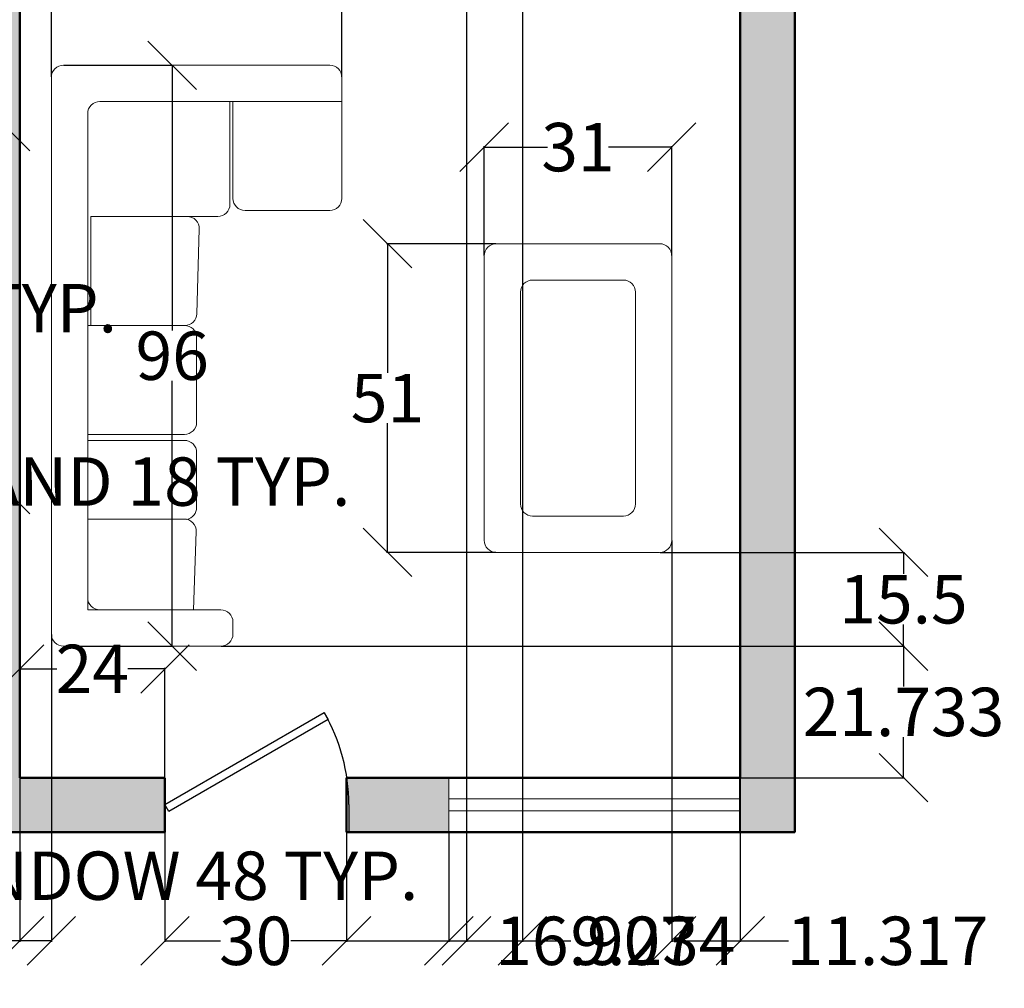
# Model space of a CAD drawing. Units: inches. Extents: x -87 to 308, y -349 to 42.
# Tile 3 of 6: x 119 to 281, y -349 to -189. Entities that reach past the tile are written whole.
import ezdxf

# ---------------------------------------------------------------- set-up
doc = ezdxf.new("R2010")
doc.units = ezdxf.units.IN
doc.header["$MEASUREMENT"] = 0
for name, color, linetype, lineweight in [('A-ANNO-DIMS', 2, 'Continuous', 18), ('A-DOOR', 3, 'Continuous', 25), ('A-FURN', 8, 'Continuous', 18), ('A-GLAZ', 4, 'Continuous', 18), ('A-WALL', 7, 'Continuous', 50), ('A-WALL-PATT', 251, 'Continuous', 13)]:
    doc.layers.add(name, color=color, linetype=linetype, lineweight=lineweight)
doc.styles.get("Standard").update_dxf_attribs({"font": 'arial.ttf'})
doc.dimstyles.get("Standard").update_dxf_attribs({"dimtxt": 8, "dimasz": 8, "dimexe": 0.18, "dimexo": 0.0625, "dimgap": 0.09, "dimtad": 0, "dimtih": 1, "dimtoh": 1, "dimdec": 0, "dimzin": 0, "dimdsep": 46, "dimlunit": 4, "dimtxsty": 'Standard', "dimblk": 'OBLIQUE', "dimcen": 0.09, "dimadec": 0, "dimazin": 0, "dimtfac": 1, "dimtdec": 0, "dimtofl": 0, "dimtmove": 0, "dimatfit": 3, "dimldrblk": 'OBLIQUE', "dimfxl": 1, "dimtolj": 1, "dimtzin": 0, "dimarcsym": 0})

# ---------------------------------------------------------------- blocks, each defined once
blk = doc.blocks.new('*U4')
for p, q in [((0, 0), (0, -6)), ((40, 0), (40, -6))]:
    blk.add_line(p, q)
blk.add_lwpolyline([(0, 0), (34.64, 20), (35.52, 18.48), (0.87, -1.52)], close=True)
blk.add_arc((0, 0), 40, 0, 30)
blk = doc.blocks.new('WIN-48IN')
for p, q in [((0, 5.5), (48, 5.5)), ((0, 3.5), (48, 3.5))]:
    blk.add_line(p, q)
for points in [[(0, 0), (0, 9)], [(48, 9), (48, 0)]]:
    blk.add_lwpolyline(points)
blk = doc.blocks.new('_Oblique')
at = {"color": 0, "linetype": 'ByBlock', "lineweight": -2}
blk.add_line((-0.5, -0.5), (0.5, 0.5), dxfattribs=at)
blk = doc.blocks.new('*D23')
at = {"layer": 'A-ANNO-DIMS', "color": 0, "lineweight": -2, "transparency": 16777216}
for p, q in [((40.22, -323.73), (40.22, -331.05)), ((88.22, -323.73), (88.22, -331.05)), ((40.22, -330.87), (88.22, -330.87)), ((88.22, -330.87), (96.22, -330.87))]:
    blk.add_line(p, q, dxfattribs=at)
at = {"layer": 'Defpoints', "color": 0, "transparency": 16777216}
for p in [(40.22, -323.67), (88.22, -323.67), (88.22, -330.87)]:
    blk.add_point(p, dxfattribs=at)
at = {"layer": 'A-ANNO-DIMS', "color": 0, "lineweight": -2, "transparency": 16777216, "xscale": 8, "yscale": 8, "zscale": 8, "rotation": 180}
blk.add_blockref('_Oblique', (40.22, -330.87), dxfattribs=at)
at = {"layer": 'A-ANNO-DIMS', "color": 0, "lineweight": -2, "transparency": 16777216, "xscale": 8, "yscale": 8, "zscale": 8}
blk.add_blockref('_Oblique', (88.22, -330.87), dxfattribs=at)
at = {"layer": 'A-ANNO-DIMS', "color": 0, "transparency": 16777216, "insert": (142.01, -330.87), "char_height": 8, "attachment_point": 5}
blk.add_mtext('\\A1;WINDOW 48 TYP.', dxfattribs=at)
blk = doc.blocks.new('*D30')
at = {"layer": 'A-ANNO-DIMS', "color": 0, "lineweight": -2, "transparency": 16777216}
for p, q in [((104.43, -207.09), (116.55, -207.09)), ((116.37, -207.09), (116.37, -232.92)), ((116.37, -267.09), (116.37, -241.27)), ((104.43, -267.09), (116.55, -267.09))]:
    blk.add_line(p, q, dxfattribs=at)
at = {"layer": 'Defpoints', "color": 0, "transparency": 16777216}
for p in [(104.37, -207.09), (116.37, -207.09), (104.37, -267.09)]:
    blk.add_point(p, dxfattribs=at)
at = {"layer": 'A-ANNO-DIMS', "color": 0, "lineweight": -2, "transparency": 16777216, "xscale": 8, "yscale": 8, "zscale": 8}
for p, rotation in [((116.37, -207.09), 90), ((116.37, -267.09), 270)]:
    blk.add_blockref('_Oblique', p, dxfattribs=dict(at, rotation=rotation))
at = {"layer": 'A-ANNO-DIMS', "color": 0, "transparency": 16777216, "insert": (116.37, -237.09), "char_height": 8, "attachment_point": 5}
blk.add_mtext('\\A1;60 TYP.', dxfattribs=at)
blk = doc.blocks.new('*D35')
at = {"layer": 'A-ANNO-DIMS', "color": 0, "lineweight": -2, "transparency": 16777216}
for p, q in [((24.45, -268.37), (24.45, -265.56)), ((24.45, -265.74), (42.45, -265.74)), ((42.45, -268.37), (42.45, -265.56)), ((42.45, -265.74), (50.45, -265.74))]:
    blk.add_line(p, q, dxfattribs=at)
at = {"layer": 'Defpoints', "color": 0, "transparency": 16777216}
for p in [(42.45, -265.74), (24.45, -268.44), (42.45, -268.44)]:
    blk.add_point(p, dxfattribs=at)
at = {"layer": 'A-ANNO-DIMS', "color": 0, "lineweight": -2, "transparency": 16777216, "xscale": 8, "yscale": 8, "zscale": 8, "rotation": 180}
blk.add_blockref('_Oblique', (24.45, -265.74), dxfattribs=at)
at = {"layer": 'A-ANNO-DIMS', "color": 0, "lineweight": -2, "transparency": 16777216, "xscale": 8, "yscale": 8, "zscale": 8}
blk.add_blockref('_Oblique', (42.45, -265.74), dxfattribs=at)
at = {"layer": 'A-ANNO-DIMS', "color": 0, "transparency": 16777216, "insert": (113.92, -265.74), "char_height": 8, "attachment_point": 5}
blk.add_mtext('\\A1;L. NIGHTSTAND 18 TYP.', dxfattribs=at)
blk = doc.blocks.new('*D52')
at = {"layer": 'A-ANNO-DIMS', "color": 0, "lineweight": -2, "transparency": 16777216}
for p, q in [((118.71, -314.61), (118.71, -296.52)), ((118.71, -296.7), (124.84, -296.7)), ((142.71, -296.7), (136.58, -296.7)), ((142.71, -314.61), (142.71, -296.52))]:
    blk.add_line(p, q, dxfattribs=at)
at = {"layer": 'Defpoints', "color": 0, "transparency": 16777216}
for p in [(142.71, -296.7), (118.71, -314.67), (142.71, -314.67)]:
    blk.add_point(p, dxfattribs=at)
at = {"layer": 'A-ANNO-DIMS', "color": 0, "lineweight": -2, "transparency": 16777216, "xscale": 8, "yscale": 8, "zscale": 8, "rotation": 180}
blk.add_blockref('_Oblique', (118.71, -296.7), dxfattribs=at)
at = {"layer": 'A-ANNO-DIMS', "color": 0, "lineweight": -2, "transparency": 16777216, "xscale": 8, "yscale": 8, "zscale": 8}
blk.add_blockref('_Oblique', (142.71, -296.7), dxfattribs=at)
at = {"layer": 'A-ANNO-DIMS', "color": 0, "transparency": 16777216, "insert": (130.71, -296.7), "char_height": 8, "attachment_point": 5}
blk.add_mtext('\\A1;24', dxfattribs=at)
blk = doc.blocks.new('*D53')
at = {"layer": 'A-ANNO-DIMS', "color": 0, "lineweight": -2, "transparency": 16777216}
for p, q in [((142.71, -323.73), (142.71, -341.81)), ((172.71, -323.73), (172.71, -341.81)), ((142.71, -341.63), (151.91, -341.63)), ((172.71, -341.63), (163.52, -341.63))]:
    blk.add_line(p, q, dxfattribs=at)
at = {"layer": 'Defpoints', "color": 0, "transparency": 16777216}
for p in [(142.71, -323.67), (172.71, -323.67), (172.71, -341.63)]:
    blk.add_point(p, dxfattribs=at)
at = {"layer": 'A-ANNO-DIMS', "color": 0, "lineweight": -2, "transparency": 16777216, "xscale": 8, "yscale": 8, "zscale": 8, "rotation": 180}
blk.add_blockref('_Oblique', (142.71, -341.63), dxfattribs=at)
at = {"layer": 'A-ANNO-DIMS', "color": 0, "lineweight": -2, "transparency": 16777216, "xscale": 8, "yscale": 8, "zscale": 8}
blk.add_blockref('_Oblique', (172.71, -341.63), dxfattribs=at)
at = {"layer": 'A-ANNO-DIMS', "color": 0, "transparency": 16777216, "insert": (157.71, -341.63), "char_height": 8, "attachment_point": 5}
blk.add_mtext('\\A1;30', dxfattribs=at)
blk = doc.blocks.new('*D54')
at = {"layer": 'A-ANNO-DIMS', "color": 0, "lineweight": -2, "transparency": 16777216}
for p, q in [((172.71, -323.73), (172.71, -341.81)), ((189.62, -323.73), (189.62, -341.81)), ((172.71, -341.63), (189.62, -341.63)), ((189.62, -341.63), (197.62, -341.63))]:
    blk.add_line(p, q, dxfattribs=at)
at = {"layer": 'Defpoints', "color": 0, "transparency": 16777216}
for p in [(172.71, -323.67), (189.62, -323.67), (189.62, -341.63)]:
    blk.add_point(p, dxfattribs=at)
at = {"layer": 'A-ANNO-DIMS', "color": 0, "lineweight": -2, "transparency": 16777216, "xscale": 8, "yscale": 8, "zscale": 8, "rotation": 180}
blk.add_blockref('_Oblique', (172.71, -341.63), dxfattribs=at)
at = {"layer": 'A-ANNO-DIMS', "color": 0, "lineweight": -2, "transparency": 16777216, "xscale": 8, "yscale": 8, "zscale": 8}
blk.add_blockref('_Oblique', (189.62, -341.63), dxfattribs=at)
at = {"layer": 'A-ANNO-DIMS', "color": 0, "transparency": 16777216, "insert": (213.94, -341.63), "char_height": 8, "attachment_point": 5}
blk.add_mtext('\\A1;16.907', dxfattribs=at)
blk = doc.blocks.new('*D77')
at = {"layer": 'A-ANNO-DIMS', "color": 0, "lineweight": -2, "transparency": 16777216}
for p, q in [((123.95, -198.87), (123.95, -180.79)), ((123.95, -180.97), (141.96, -180.97)), ((171.95, -180.97), (153.94, -180.97)), ((171.95, -198.87), (171.95, -180.79))]:
    blk.add_line(p, q, dxfattribs=at)
at = {"layer": 'Defpoints', "color": 0, "transparency": 16777216}
for p in [(171.95, -180.97), (123.95, -198.94), (171.95, -198.94)]:
    blk.add_point(p, dxfattribs=at)
at = {"layer": 'A-ANNO-DIMS', "color": 0, "lineweight": -2, "transparency": 16777216, "xscale": 8, "yscale": 8, "zscale": 8, "rotation": 180}
blk.add_blockref('_Oblique', (123.95, -180.97), dxfattribs=at)
at = {"layer": 'A-ANNO-DIMS', "color": 0, "lineweight": -2, "transparency": 16777216, "xscale": 8, "yscale": 8, "zscale": 8}
blk.add_blockref('_Oblique', (171.95, -180.97), dxfattribs=at)
at = {"layer": 'A-ANNO-DIMS', "color": 0, "transparency": 16777216, "insert": (147.95, -180.97), "char_height": 8, "attachment_point": 5}
blk.add_mtext('\\A1;48', dxfattribs=at)
blk = doc.blocks.new('*D78')
at = {"layer": 'A-ANNO-DIMS', "color": 0, "lineweight": -2, "transparency": 16777216}
for p, q in [((126.01, -196.94), (144.09, -196.94)), ((143.91, -196.94), (143.91, -240.76)), ((143.91, -292.94), (143.91, -249.11)), ((126.01, -292.94), (144.09, -292.94))]:
    blk.add_line(p, q, dxfattribs=at)
at = {"layer": 'Defpoints', "color": 0, "transparency": 16777216}
for p in [(125.95, -196.94), (125.95, -292.94), (143.91, -292.94)]:
    blk.add_point(p, dxfattribs=at)
at = {"layer": 'A-ANNO-DIMS', "color": 0, "lineweight": -2, "transparency": 16777216, "xscale": 8, "yscale": 8, "zscale": 8}
for p, rotation in [((143.91, -196.94), 90), ((143.91, -292.94), 270)]:
    blk.add_blockref('_Oblique', p, dxfattribs=dict(at, rotation=rotation))
at = {"layer": 'A-ANNO-DIMS', "color": 0, "transparency": 16777216, "insert": (143.91, -244.94), "char_height": 8, "attachment_point": 5}
blk.add_mtext('\\A1;96', dxfattribs=at)
blk = doc.blocks.new('*D79')
at = {"layer": 'A-ANNO-DIMS', "color": 0, "lineweight": -2, "transparency": 16777216}
for p, q in [((195.45, -228.37), (195.45, -210.29)), ((195.45, -210.47), (205.9, -210.47)), ((226.45, -210.47), (215.99, -210.47)), ((226.45, -228.37), (226.45, -210.29))]:
    blk.add_line(p, q, dxfattribs=at)
at = {"layer": 'Defpoints', "color": 0, "transparency": 16777216}
for p in [(226.45, -210.47), (195.45, -228.44), (226.45, -228.44)]:
    blk.add_point(p, dxfattribs=at)
at = {"layer": 'A-ANNO-DIMS', "color": 0, "lineweight": -2, "transparency": 16777216, "xscale": 8, "yscale": 8, "zscale": 8, "rotation": 180}
blk.add_blockref('_Oblique', (195.45, -210.47), dxfattribs=at)
at = {"layer": 'A-ANNO-DIMS', "color": 0, "lineweight": -2, "transparency": 16777216, "xscale": 8, "yscale": 8, "zscale": 8}
blk.add_blockref('_Oblique', (226.45, -210.47), dxfattribs=at)
at = {"layer": 'A-ANNO-DIMS', "color": 0, "transparency": 16777216, "insert": (210.95, -210.47), "char_height": 8, "attachment_point": 5}
blk.add_mtext('\\A1;31', dxfattribs=at)
blk = doc.blocks.new('*D80')
at = {"layer": 'A-ANNO-DIMS', "color": 0, "lineweight": -2, "transparency": 16777216}
for p, q in [((197.38, -226.44), (179.3, -226.44)), ((179.48, -226.44), (179.48, -247.76)), ((179.48, -277.44), (179.48, -256.11)), ((197.38, -277.44), (179.3, -277.44))]:
    blk.add_line(p, q, dxfattribs=at)
at = {"layer": 'Defpoints', "color": 0, "transparency": 16777216}
for p in [(179.48, -226.44), (197.45, -226.44), (197.45, -277.44)]:
    blk.add_point(p, dxfattribs=at)
at = {"layer": 'A-ANNO-DIMS', "color": 0, "lineweight": -2, "transparency": 16777216, "xscale": 8, "yscale": 8, "zscale": 8}
for p, rotation in [((179.48, -226.44), 90), ((179.48, -277.44), 270)]:
    blk.add_blockref('_Oblique', p, dxfattribs=dict(at, rotation=rotation))
at = {"layer": 'A-ANNO-DIMS', "color": 0, "transparency": 16777216, "insert": (179.48, -251.94), "char_height": 8, "attachment_point": 5}
blk.add_mtext('\\A1;51', dxfattribs=at)
blk = doc.blocks.new('*D90')
at = {"layer": 'A-ANNO-DIMS', "color": 0, "lineweight": -2, "transparency": 16777216}
for p, q in [((123.95, -291), (123.95, -341.81)), ((118.71, -314.73), (118.71, -341.81)), ((118.71, -341.63), (110.71, -341.63)), ((123.95, -341.63), (118.71, -341.63))]:
    blk.add_line(p, q, dxfattribs=at)
at = {"layer": 'Defpoints', "color": 0, "transparency": 16777216}
for p in [(123.95, -290.94), (118.71, -314.67), (118.71, -341.63)]:
    blk.add_point(p, dxfattribs=at)
at = {"layer": 'A-ANNO-DIMS', "color": 0, "lineweight": -2, "transparency": 16777216, "xscale": 8, "yscale": 8, "zscale": 8, "rotation": 180}
blk.add_blockref('_Oblique', (118.71, -341.63), dxfattribs=at)
at = {"layer": 'A-ANNO-DIMS', "color": 0, "lineweight": -2, "transparency": 16777216, "xscale": 8, "yscale": 8, "zscale": 8}
blk.add_blockref('_Oblique', (123.95, -341.63), dxfattribs=at)
at = {"layer": 'A-ANNO-DIMS', "color": 0, "transparency": 16777216, "insert": (97.14, -341.63), "char_height": 8, "attachment_point": 5}
blk.add_mtext('\\A1;5.234', dxfattribs=at)
blk = doc.blocks.new('*D91')
at = {"layer": 'A-ANNO-DIMS', "color": 0, "lineweight": -2, "transparency": 16777216}
for p, q in [((152.01, -292.94), (264.91, -292.94)), ((264.73, -292.94), (264.73, -299.62)), ((264.73, -314.67), (264.73, -307.98)), ((172.78, -314.67), (264.91, -314.67))]:
    blk.add_line(p, q, dxfattribs=at)
at = {"layer": 'Defpoints', "color": 0, "transparency": 16777216}
for p in [(151.95, -292.94), (172.71, -314.67), (264.73, -314.67)]:
    blk.add_point(p, dxfattribs=at)
at = {"layer": 'A-ANNO-DIMS', "color": 0, "lineweight": -2, "transparency": 16777216, "xscale": 8, "yscale": 8, "zscale": 8}
for p, rotation in [((264.73, -292.94), 90), ((264.73, -314.67), 270)]:
    blk.add_blockref('_Oblique', p, dxfattribs=dict(at, rotation=rotation))
at = {"layer": 'A-ANNO-DIMS', "color": 0, "transparency": 16777216, "insert": (264.73, -303.8), "char_height": 8, "attachment_point": 5}
blk.add_mtext('\\A1;21.733', dxfattribs=at)
blk = doc.blocks.new('*D92')
at = {"layer": 'A-ANNO-DIMS', "color": 0, "lineweight": -2, "transparency": 16777216}
for p, q in [((226.45, -275.5), (226.45, -341.81)), ((237.76, -314.73), (237.76, -341.81)), ((226.45, -341.63), (237.76, -341.63)), ((237.76, -341.63), (245.76, -341.63))]:
    blk.add_line(p, q, dxfattribs=at)
at = {"layer": 'Defpoints', "color": 0, "transparency": 16777216}
for p in [(226.45, -275.44), (237.76, -314.67), (237.76, -341.63)]:
    blk.add_point(p, dxfattribs=at)
at = {"layer": 'A-ANNO-DIMS', "color": 0, "lineweight": -2, "transparency": 16777216, "xscale": 8, "yscale": 8, "zscale": 8, "rotation": 180}
blk.add_blockref('_Oblique', (226.45, -341.63), dxfattribs=at)
at = {"layer": 'A-ANNO-DIMS', "color": 0, "lineweight": -2, "transparency": 16777216, "xscale": 8, "yscale": 8, "zscale": 8}
blk.add_blockref('_Oblique', (237.76, -341.63), dxfattribs=at)
at = {"layer": 'A-ANNO-DIMS', "color": 0, "transparency": 16777216, "insert": (262.08, -341.63), "char_height": 8, "attachment_point": 5}
blk.add_mtext('\\A1;11.317', dxfattribs=at)
blk = doc.blocks.new('*D93')
at = {"layer": 'A-ANNO-DIMS', "color": 0, "lineweight": -2, "transparency": 16777216}
for p, q in [((224.51, -277.44), (264.91, -277.44)), ((264.73, -277.44), (264.73, -281.01)), ((264.73, -292.94), (264.73, -289.36)), ((152.01, -292.94), (264.91, -292.94))]:
    blk.add_line(p, q, dxfattribs=at)
at = {"layer": 'Defpoints', "color": 0, "transparency": 16777216}
for p in [(224.45, -277.44), (151.95, -292.94), (264.73, -292.94)]:
    blk.add_point(p, dxfattribs=at)
at = {"layer": 'A-ANNO-DIMS', "color": 0, "lineweight": -2, "transparency": 16777216, "xscale": 8, "yscale": 8, "zscale": 8}
for p, rotation in [((264.73, -277.44), 90), ((264.73, -292.94), 270)]:
    blk.add_blockref('_Oblique', p, dxfattribs=dict(at, rotation=rotation))
at = {"layer": 'A-ANNO-DIMS', "color": 0, "transparency": 16777216, "insert": (264.73, -285.19), "char_height": 8, "attachment_point": 5}
blk.add_mtext('\\A1;15.5', dxfattribs=at)
blk = doc.blocks.new('*D94')
at = {"layer": 'A-ANNO-DIMS', "color": 0, "lineweight": -2, "transparency": 16777216}
for p, q in [((192.53, -154.67), (192.53, -341.81)), ((201.76, -162.73), (201.76, -341.81)), ((192.53, -341.63), (201.76, -341.63)), ((201.76, -341.63), (209.76, -341.63))]:
    blk.add_line(p, q, dxfattribs=at)
at = {"layer": 'Defpoints', "color": 0, "transparency": 16777216}
for p in [(192.53, -154.61), (201.76, -162.67), (201.76, -341.63)]:
    blk.add_point(p, dxfattribs=at)
at = {"layer": 'A-ANNO-DIMS', "color": 0, "lineweight": -2, "transparency": 16777216, "xscale": 8, "yscale": 8, "zscale": 8, "rotation": 180}
blk.add_blockref('_Oblique', (192.53, -341.63), dxfattribs=at)
at = {"layer": 'A-ANNO-DIMS', "color": 0, "lineweight": -2, "transparency": 16777216, "xscale": 8, "yscale": 8, "zscale": 8}
blk.add_blockref('_Oblique', (201.76, -341.63), dxfattribs=at)
at = {"layer": 'A-ANNO-DIMS', "color": 0, "transparency": 16777216, "insert": (223.34, -341.63), "char_height": 8, "attachment_point": 5}
blk.add_mtext('\\A1;9.234', dxfattribs=at)

msp = doc.modelspace()

# ---------------------------------------------------------------- hatches: boundary and pattern name
at = {"layer": 'A-WALL-PATT'}
h = msp.add_hatch(color=256, dxfattribs=at)
h.dxf.hatch_style = 1
h.paths.add_polyline_path([(246.7637, -136.9351), (237.7637, -136.9351), (237.7637, -162.668), (237.7637, -166.668), (237.7637, -314.668), (237.6195, -323.668), (246.7637, -323.668)])
h = msp.add_hatch(color=256, dxfattribs=at)
h.dxf.hatch_style = 1
h.paths.add_polyline_path([(118.7127, -170.668), (118.7127, -166.668), (114.7127, -166.668), (110.7127, -166.668), (110.7127, -170.668), (114.7127, -170.668), (114.7127, -314.668), (88.2177, -314.668), (88.2177, -323.668), (142.7127, -323.668), (142.7127, -319.1107), (142.7127, -314.668), (118.7127, -314.668)])
h = msp.add_hatch(color=256, dxfattribs=at)
h.dxf.hatch_style = 1
h.paths.add_polyline_path([(189.6195, -314.668), (172.7684, -314.668, -0.03670428), (173.095, -319.1107), (173.095, -323.668), (189.6195, -323.668)])

# ---------------------------------------------------------------- linework, layer by layer
at = {"layer": 'A-FURN'}
for p, q in [((125.9465, -196.9351), (169.9465, -196.9351)), ((123.9465, -290.9351), (123.9465, -198.9351)), ((171.9465, -198.9351), (171.9465, -202.9351)), ((171.9465, -202.9351), (131.9465, -202.9351)), ((129.9465, -204.9351), (129.9465, -286.9351)), ((148.4465, -221.9351), (146.3902, -221.9351)), ((129.9465, -286.9351), (151.9465, -286.9351)), ((153.9465, -288.9351), (153.9465, -290.9351)), ((151.9465, -292.9351), (125.9465, -292.9351))]:
    msp.add_line(p, q, dxfattribs=at)
for points in [[(148.4465, -221.9351), (151.4465, -221.9351, 0.41421356), (153.4465, -219.9351), (153.4465, -202.9351), (135.4465, -202.9351)], [(146.3475, -271.9834, 0.3562473), (147.9465, -270.024), (147.9465, -260.9351, 0.41421356), (145.9465, -258.9351), (129.9465, -258.9351), (129.9465, -276.9351)]]:
    msp.add_lwpolyline(points, format="xyb", dxfattribs=at)
for points in [[(171.9465, -202.9351), (153.9465, -202.9351), (153.9465, -218.9351, 0.41421356), (155.9465, -220.9351), (169.9465, -220.9351, 0.41421356), (171.9465, -218.9351)], [(146.3902, -221.9351), (130.4465, -221.9351), (130.4465, -239.9351), (146.0013, -239.9351, 0.40610293), (148.0005, -237.9906), (148.3894, -223.9906, 0.42237098)], [(197.4465, -226.4351), (224.4465, -226.4351, -0.41421356), (226.4465, -228.4351), (226.4465, -275.4351, -0.41421356), (224.4465, -277.4351), (197.4465, -277.4351, -0.41421356), (195.4465, -275.4351), (195.4465, -228.4351, -0.41421356)], [(203.4465, -232.4351), (218.4465, -232.4351, -0.41421356), (220.4465, -234.4351), (220.4465, -269.4351, -0.41421356), (218.4465, -271.4351), (203.4465, -271.4351, -0.41421356), (201.4465, -269.4351), (201.4465, -234.4351, -0.41421356)], [(145.9465, -239.9351), (129.9465, -239.9351), (129.9465, -257.9351), (145.9465, -257.9351, 0.41421356), (147.9465, -255.9351), (147.9465, -241.9351, 0.41421356)], [(129.9465, -271.9351), (145.8781, -271.9277, -0.42414348), (147.8779, -273.9944), (147.4468, -286.9268), (131.9475, -286.9342, -0.41435289), (129.9465, -284.9342)]]:
    msp.add_lwpolyline(points, format="xyb", close=True, dxfattribs=at)
for centre, start, end in [((125.9465, -198.9351), 90, 180), ((169.9465, -198.9351), 0, 90), ((131.9465, -204.9351), 90, 180), ((151.9465, -288.9351), 0, 90), ((125.9465, -290.9351), 180, 270), ((151.9465, -290.9351), 270, 0)]:
    msp.add_arc(centre, 2, start, end, dxfattribs=at)
at = {"layer": 'A-WALL'}
for p, q in [((237.7637, -166.668), (237.7637, -314.668)), ((118.7127, -170.668), (118.7127, -314.668)), ((142.7127, -314.668), (118.7127, -314.668)), ((142.7127, -314.668), (142.7127, -323.668)), ((237.7637, -314.668), (172.7127, -314.668)), ((172.7127, -314.668), (172.7127, -323.668))]:
    msp.add_line(p, q, dxfattribs=at)
msp.add_lwpolyline([(142.7127, -323.668), (12.7637, -323.668), (12.7637, 18.332), (246.7637, 18.332), (246.7637, -323.668), (172.7127, -323.668)], dxfattribs=at)

# ---------------------------------------------------------------- block references
at = {"layer": 'A-DOOR', "xscale": 0.7595575434647344, "yscale": 0.7595575434647344, "zscale": 0.7595575434647344}
msp.add_blockref('*U4', (142.7127, -319.1107), dxfattribs=at)
at = {"layer": 'A-GLAZ'}
msp.add_blockref('WIN-48IN', (189.6194, -323.668), dxfattribs=at)

# ---------------------------------------------------------------- dimensions: what is measured, and where the dimension line sits
at = {"layer": 'A-ANNO-DIMS'}
for base, p1, p2, override, picture, middle in [((201.7637, -341.6325), (192.5294, -154.6053), (201.7637, -162.668), {"dimdec": 3, "dimlfac": 1, "dimrnd": 0, "dimzin": 0, "dimdsep": 46, "dimlunit": 2}, '*D94', (223.3352, -341.6325)), ((171.9465, -180.9706), (123.9465, -198.9351), (171.9465, -198.9351), {"dimdec": 0, "dimlfac": 1, "dimrnd": 0, "dimzin": 0, "dimdsep": 46, "dimlunit": 2}, '*D77', (147.9465, -180.9706)), ((226.4465, -210.4706), (195.4465, -228.4351), (226.4465, -228.4351), {"dimdec": 0, "dimlfac": 1, "dimrnd": 0, "dimzin": 0, "dimdsep": 46, "dimlunit": 2}, '*D79', (210.9465, -210.4706)), ((237.7637, -341.6325), (226.4465, -275.4351), (237.7637, -314.668), {"dimdec": 3, "dimlfac": 1, "dimrnd": 0, "dimzin": 0, "dimdsep": 46, "dimlunit": 2}, '*D92', (262.0829, -341.6325)), ((118.7127, -341.6325), (123.9465, -290.9351), (118.7127, -314.668), {"dimdec": 3, "dimlfac": 1, "dimrnd": 0, "dimzin": 0, "dimdsep": 46, "dimlunit": 2}, '*D90', (97.1411, -341.6325)), ((142.7127, -296.7035), (118.7127, -314.668), (142.7127, -314.668), {"dimdec": 0, "dimlfac": 1, "dimrnd": 0, "dimzin": 0, "dimdsep": 46, "dimlunit": 2}, '*D52', (130.7127, -296.7035)), ((172.7127, -341.6325), (142.7127, -323.668), (172.7127, -323.668), {"dimdec": 0, "dimlfac": 1, "dimrnd": 0, "dimzin": 0, "dimdsep": 46, "dimlunit": 2}, '*D53', (157.7127, -341.6325)), ((189.6195, -341.6325), (172.7127, -323.668), (189.6195, -323.668), {"dimdec": 3, "dimlfac": 1, "dimrnd": 0, "dimzin": 0, "dimdsep": 46, "dimlunit": 2}, '*D54', (213.9387, -341.6325))]:
    dim = msp.add_linear_dim(base=base, p1=p1, p2=p2, dimstyle='Standard', override=override, dxfattribs=at)
    dim.commit()
    dim.dimension.update_dxf_attribs({"geometry": picture, "text_midpoint": middle})
for base, p1, p2, angle, override, picture, middle in [((143.911, -292.9351), (125.9465, -196.9351), (125.9465, -292.9351), 270, {"dimdec": 0, "dimlfac": 1, "dimrnd": 0, "dimzin": 0, "dimdsep": 46, "dimlunit": 2}, '*D78', (143.911, -244.9351)), ((179.482, -226.4351), (197.4465, -277.4351), (197.4465, -226.4351), 90, {"dimdec": 0, "dimlfac": 1, "dimrnd": 0, "dimzin": 0, "dimdsep": 46, "dimlunit": 2}, '*D80', (179.482, -251.9351)), ((264.7282, -292.9351), (224.4465, -277.4351), (151.9465, -292.9351), 90, {"dimdec": 1, "dimlfac": 1, "dimrnd": 0, "dimzin": 0, "dimdsep": 46, "dimlunit": 2}, '*D93', (264.7282, -285.1851)), ((264.7282, -314.668), (151.9465, -292.9351), (172.7127, -314.668), 90, {"dimdec": 3, "dimlfac": 1, "dimrnd": 0, "dimzin": 0, "dimdsep": 46, "dimlunit": 2}, '*D91', (264.7282, -303.8016))]:
    dim = msp.add_linear_dim(base=base, p1=p1, p2=p2, angle=angle, dimstyle='Standard', override=override, dxfattribs=at)
    dim.commit()
    dim.dimension.update_dxf_attribs({"geometry": picture, "text_midpoint": middle})
dim = msp.add_linear_dim(base=(116.3666, -207.0911), p1=(104.3666, -267.0911), p2=(104.3666, -207.0911), angle=90, text='<> TYP.', dimstyle='Standard', override={"dimdec": 0, "dimlfac": 1, "dimrnd": 0, "dimzin": 0, "dimdsep": 46, "dimlunit": 2}, dxfattribs=at)
dim.commit()
dim.dimension.update_dxf_attribs({"geometry": '*D30', "text_midpoint": (116.3666, -237.0911)})
for base, p1, p2, text, picture, middle in [((42.4465, -265.7351), (24.4465, -268.4351), (42.4465, -268.4351), 'L. NIGHTSTAND <> TYP.', '*D35', (113.9171, -265.7351)), ((88.2177, -330.868), (40.2177, -323.668), (88.2177, -323.668), 'WINDOW <> TYP.', '*D23', (142.013, -330.868))]:
    dim = msp.add_linear_dim(base=base, p1=p1, p2=p2, text=text, dimstyle='Standard', override={"dimdec": 0, "dimlfac": 1, "dimrnd": 0, "dimzin": 0, "dimdsep": 46, "dimlunit": 2}, dxfattribs=at)
    dim.commit()
    dim.dimension.update_dxf_attribs({"geometry": picture, "text_midpoint": middle})

doc.saveas('drawing.dxf')
